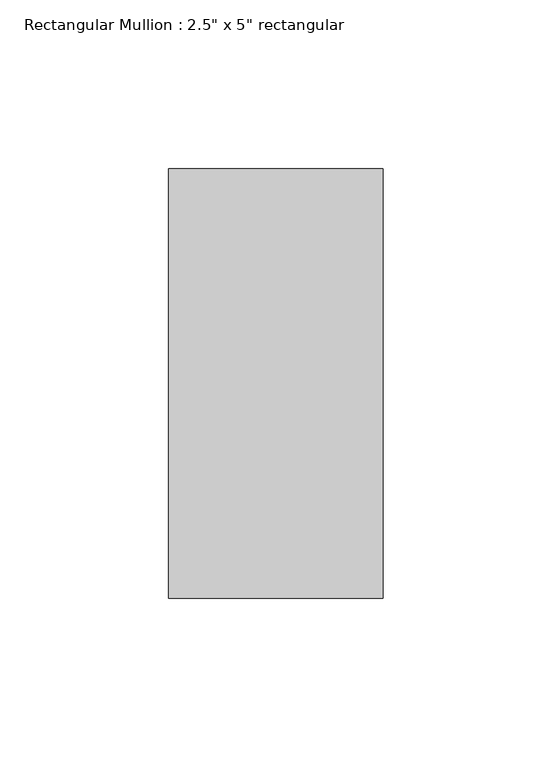
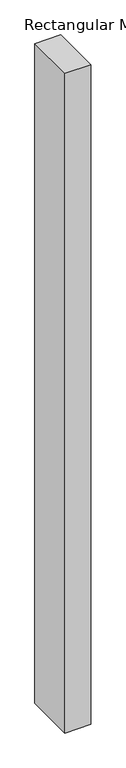
"""IFC4 building model written with IfcOpenShell, lengths in millimetres: member geometry."""

from ifc_helpers import new_model, si_unit, frame, origin, place, context, project, spatial, polyline, outline, extrude, source, transform, mapped, element, save


def member_17644e48(model_context):
    return source(origin(), model_context, "Body", "SweptSolid", [
        extrude(outline(polyline([(0.0, 63.5), (0.0, -63.5), (-63.5, -63.5), (-63.5, 63.5), (0.0, 63.5)])), frame((0.0, 0.0, -1707.486558), z_axis=(0.0, 0.0, 1.0), x_axis=(1.0, 0.0, 0.0)), (0.0, 0.0, 1.0), 1707.486558),
    ])


if __name__ == "__main__":
    model = new_model("IFC4")
    model_context = context("Model", 3, world=origin())
    ifc_project = project(units=[si_unit("LENGTHUNIT", "METRE", prefix="MILLI")], contexts=[model_context])
    site = spatial("IfcSite", under=ifc_project)
    building = spatial("IfcBuilding", under=site)
    placement = place(None, origin())
    member_shape = member_17644e48(model_context)
    element("IfcMember", 1, ObjectType="Rectangular Mullion : 2.5\" x 5\" rectangular", at=placement, inside=building, context=model_context, shape_type="MappedRepresentation", body=[
        mapped(member_shape, transform((0.0, 0.0, 0.0), x_axis=(1.0, 0.0, 0.0), y_axis=(0.0, 1.0, 0.0), z_axis=(0.0, 0.0, 1.0))),
    ])
    save(model, "model.ifc")

# Revit data of these elements
# Type "Rectangular Mullion : 2.5\" x 5\" rectangular"
#   built-in parameter 1007304 = 0.416667 (stored number, unit not read)
#   built-in parameter 1007301 = 0.104167 (stored number, unit not read)
#   built-in parameter 1007300 = 0.104167 (stored number, unit not read)
# Element 1 (IfcMember, "Rectangular Mullion : 2.5\" x 5\" rectangular")
#   Materials on its faces: "Aluminum"
# Materials
#   "Aluminum": class "Metal", colour RGB 247 247 247, transparency 0, Description = "Aluminum 6061", Cost = 0
